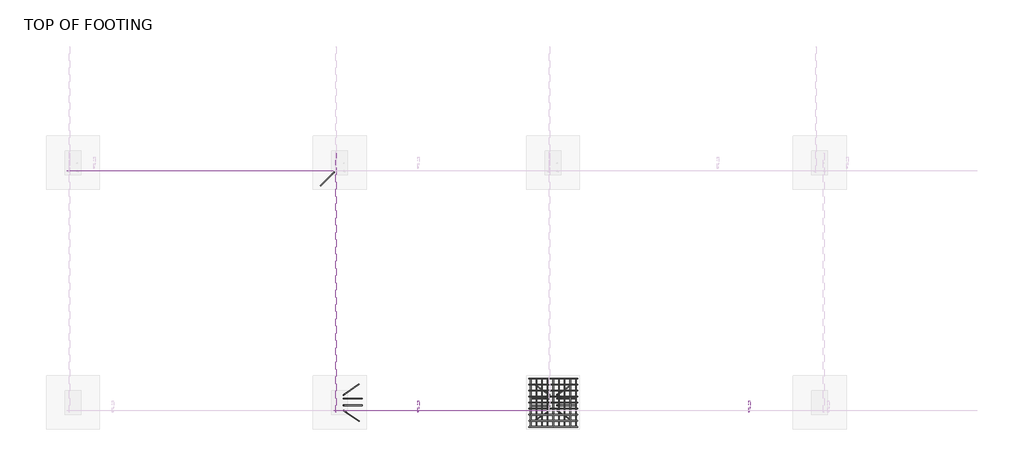
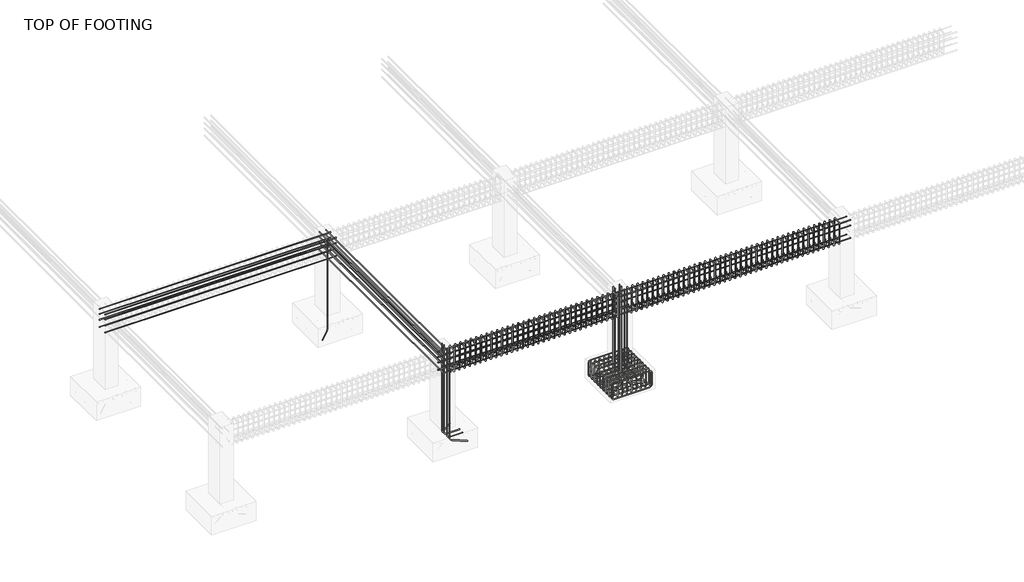
# One storey, part 3 of 13: 31 reinforcing bars.
"""IFC4 building model written with IfcOpenShell, lengths in millimetres."""

from ifc_helpers import new_model, si_unit, point, frame, origin, place, context, project, spatial, polyline, circle_curve, trimmed, segment, composite_curve, source, transform, mapped, element, save
from ifc_brep_helpers import swept_disk

model = new_model("IFC4")

# Units and contexts
model_context = context("Model", 3, world=origin())
ifc_project = project(units=[si_unit("LENGTHUNIT", "METRE", prefix="MILLI")], contexts=[model_context])

# Site, building, storey
site = spatial("IfcSite", under=ifc_project)
building = spatial("IfcBuilding", under=site)
storey = spatial("IfcBuildingStorey", under=building, Name="TOP OF FOOTING", Elevation=-1828.8)

# Reinforcing bars
placement = place(None, origin())
reinforcing_bar_shape = source(origin(), model_context, "Body", "SolidModel", [
    swept_disk(composite_curve([segment(polyline([(-3666.6498378, 3986.1851908, -2049.322685), (-3666.6498378, 3986.1851908, -2196.622685)]), True, "CONTINUOUS"), segment(trimmed(circle_curve(frame((-3712.9998378, 3986.1851908, -2196.622685), z_axis=(0.0, 1.0, 0.0), x_axis=(46.34999999999991, 0.0, 0.0)), 46.35), [point((-3666.6498378, 3986.1851908, -2196.622685))], [point((-3712.9998378, 3986.1851908, -2242.972685))], True, "CARTESIAN"), True, "CONTINUOUS"), segment(polyline([(-3712.9998378, 3986.1851908, -2242.972685), (-4527.5998378, 3986.1851908, -2242.972685)]), True, "CONTINUOUS"), segment(trimmed(circle_curve(frame((-4527.5998378, 3986.1851908, -2196.622685), z_axis=(0.0, 1.0, 0.0), x_axis=(0.0, 0.0, -46.350000000000364)), 46.35), [point((-4527.5998378, 3986.1851908, -2242.972685))], [point((-4573.9498378, 3986.1851908, -2196.622685))], True, "CARTESIAN"), True, "CONTINUOUS"), segment(polyline([(-4573.9498378, 3986.1851908, -2196.622685), (-4573.9498378, 3986.1851908, -2049.322685)]), True, "CONTINUOUS")], self_intersect=False), 6.35),
])
element("IfcReinforcingBar", 1, at=placement, inside=storey, context=model_context, shape_type="MappedRepresentation", body=[
    mapped(reinforcing_bar_shape, transform((0.0, 0.0, 0.0), x_axis=(1.0, 0.0, 0.0), y_axis=(0.0, 1.0, 0.0), z_axis=(0.0, 0.0, 1.0))),
    mapped(reinforcing_bar_shape, transform((0.0, -113.4125, 0.0), x_axis=(1.0, 0.0, 0.0), y_axis=(0.0, 1.0, 0.0), z_axis=(0.0, 0.0, 1.0))),
    mapped(reinforcing_bar_shape, transform((0.0, -226.825, 0.0), x_axis=(1.0, 0.0, 0.0), y_axis=(0.0, 1.0, 0.0), z_axis=(0.0, 0.0, 1.0))),
    mapped(reinforcing_bar_shape, transform((0.0, -340.2375, 0.0), x_axis=(1.0, 0.0, 0.0), y_axis=(0.0, 1.0, 0.0), z_axis=(0.0, 0.0, 1.0))),
    mapped(reinforcing_bar_shape, transform((0.0, -453.65, 0.0), x_axis=(1.0, 0.0, 0.0), y_axis=(0.0, 1.0, 0.0), z_axis=(0.0, 0.0, 1.0))),
    mapped(reinforcing_bar_shape, transform((0.0, -567.0625, 0.0), x_axis=(1.0, 0.0, 0.0), y_axis=(0.0, 1.0, 0.0), z_axis=(0.0, 0.0, 1.0))),
    mapped(reinforcing_bar_shape, transform((0.0, -680.475, 0.0), x_axis=(1.0, 0.0, 0.0), y_axis=(0.0, 1.0, 0.0), z_axis=(0.0, 0.0, 1.0))),
    mapped(reinforcing_bar_shape, transform((0.0, -793.8875, 0.0), x_axis=(1.0, 0.0, 0.0), y_axis=(0.0, 1.0, 0.0), z_axis=(0.0, 0.0, 1.0))),
    mapped(reinforcing_bar_shape, transform((0.0, -907.3, 0.0), x_axis=(1.0, 0.0, 0.0), y_axis=(0.0, 1.0, 0.0), z_axis=(0.0, 0.0, 1.0))),
])
reinforcing_bar_2_shape = source(origin(), model_context, "Body", "SolidModel", [
    swept_disk(composite_curve([segment(polyline([(-4573.9498378, 3986.1851908, -2051.3998363), (-4573.9498378, 3986.1851908, -1904.0998363)]), True, "CONTINUOUS"), segment(trimmed(circle_curve(frame((-4527.5998378, 3986.1851908, -1904.0998363), z_axis=(0.0, 1.0, 0.0), x_axis=(-46.349999999999454, 0.0, 0.0)), 46.35), [point((-4573.9498378, 3986.1851908, -1904.0998363))], [point((-4527.5998378, 3986.1851908, -1857.7498363))], True, "CARTESIAN"), True, "CONTINUOUS"), segment(polyline([(-4527.5998378, 3986.1851908, -1857.7498363), (-3712.9998378, 3986.1851908, -1857.7498363)]), True, "CONTINUOUS"), segment(trimmed(circle_curve(frame((-3712.9998378, 3986.1851908, -1904.0998363), z_axis=(0.0, 1.0, 0.0), x_axis=(0.0, 0.0, 46.350000000000136)), 46.35), [point((-3712.9998378, 3986.1851908, -1857.7498363))], [point((-3666.6498378, 3986.1851908, -1904.0998363))], True, "CARTESIAN"), True, "CONTINUOUS"), segment(polyline([(-3666.6498378, 3986.1851908, -1904.0998363), (-3666.6498378, 3986.1851908, -2051.3998363)]), True, "CONTINUOUS")], self_intersect=False), 6.35),
])
element("IfcReinforcingBar", 2, at=placement, inside=storey, context=model_context, shape_type="MappedRepresentation", body=[
    mapped(reinforcing_bar_2_shape, transform((0.0, 0.0, 0.0), x_axis=(1.0, 0.0, 0.0), y_axis=(0.0, 1.0, 0.0), z_axis=(0.0, 0.0, 1.0))),
    mapped(reinforcing_bar_2_shape, transform((0.0, -113.4125, 0.0), x_axis=(1.0, 0.0, 0.0), y_axis=(0.0, 1.0, 0.0), z_axis=(0.0, 0.0, 1.0))),
    mapped(reinforcing_bar_2_shape, transform((0.0, -226.825, 0.0), x_axis=(1.0, 0.0, 0.0), y_axis=(0.0, 1.0, 0.0), z_axis=(0.0, 0.0, 1.0))),
    mapped(reinforcing_bar_2_shape, transform((0.0, -340.2375, 0.0), x_axis=(1.0, 0.0, 0.0), y_axis=(0.0, 1.0, 0.0), z_axis=(0.0, 0.0, 1.0))),
    mapped(reinforcing_bar_2_shape, transform((0.0, -453.65, 0.0), x_axis=(1.0, 0.0, 0.0), y_axis=(0.0, 1.0, 0.0), z_axis=(0.0, 0.0, 1.0))),
    mapped(reinforcing_bar_2_shape, transform((0.0, -567.0625, 0.0), x_axis=(1.0, 0.0, 0.0), y_axis=(0.0, 1.0, 0.0), z_axis=(0.0, 0.0, 1.0))),
    mapped(reinforcing_bar_2_shape, transform((0.0, -680.475, 0.0), x_axis=(1.0, 0.0, 0.0), y_axis=(0.0, 1.0, 0.0), z_axis=(0.0, 0.0, 1.0))),
    mapped(reinforcing_bar_2_shape, transform((0.0, -793.8875, 0.0), x_axis=(1.0, 0.0, 0.0), y_axis=(0.0, 1.0, 0.0), z_axis=(0.0, 0.0, 1.0))),
    mapped(reinforcing_bar_2_shape, transform((0.0, -907.3, 0.0), x_axis=(1.0, 0.0, 0.0), y_axis=(0.0, 1.0, 0.0), z_axis=(0.0, 0.0, 1.0))),
])
reinforcing_bar_3_shape = source(origin(), model_context, "Body", "SolidModel", [
    swept_disk(composite_curve([segment(polyline([(-4542.4641345, 3986.1851908, -2025.081839), (-4542.4641345, 3986.1851908, -2172.381839)]), True, "CONTINUOUS"), segment(trimmed(circle_curve(frame((-4542.4641345, 3939.8351908, -2172.381839), z_axis=(-1.0, 0.0, 0.0), x_axis=(0.0, 46.34999999999991, 0.0)), 46.35), [point((-4542.4641345, 3986.1851908, -2172.381839))], [point((-4542.4641345, 3939.8351908, -2218.731839))], True, "CARTESIAN"), True, "CONTINUOUS"), segment(polyline([(-4542.4641345, 3939.8351908, -2218.731839), (-4542.4641345, 3125.2351908, -2218.731839)]), True, "CONTINUOUS"), segment(trimmed(circle_curve(frame((-4542.4641345, 3125.2351908, -2172.381839), z_axis=(-1.0, 0.0, 0.0), x_axis=(0.0, 0.0, -46.34999999999991)), 46.35), [point((-4542.4641345, 3125.2351908, -2218.731839))], [point((-4542.4641345, 3078.8851908, -2172.381839))], True, "CARTESIAN"), True, "CONTINUOUS"), segment(polyline([(-4542.4641345, 3078.8851908, -2172.381839), (-4542.4641345, 3078.8851908, -2025.081839)]), True, "CONTINUOUS")], self_intersect=False), 6.35),
])
element("IfcReinforcingBar", 3, at=placement, inside=storey, context=model_context, shape_type="MappedRepresentation", body=[
    mapped(reinforcing_bar_3_shape, transform((0.0, 0.0, 0.0), x_axis=(1.0, 0.0, 0.0), y_axis=(0.0, 1.0, 0.0), z_axis=(0.0, 0.0, 1.0))),
    mapped(reinforcing_bar_3_shape, transform((105.924033, 0.0, 0.0), x_axis=(1.0, 0.0, 0.0), y_axis=(0.0, 1.0, 0.0), z_axis=(0.0, 0.0, 1.0))),
    mapped(reinforcing_bar_3_shape, transform((211.8480661, 0.0, 0.0), x_axis=(1.0, 0.0, 0.0), y_axis=(0.0, 1.0, 0.0), z_axis=(0.0, 0.0, 1.0))),
    mapped(reinforcing_bar_3_shape, transform((317.7720991, 0.0, 0.0), x_axis=(1.0, 0.0, 0.0), y_axis=(0.0, 1.0, 0.0), z_axis=(0.0, 0.0, 1.0))),
    mapped(reinforcing_bar_3_shape, transform((423.6961321, 0.0, 0.0), x_axis=(1.0, 0.0, 0.0), y_axis=(0.0, 1.0, 0.0), z_axis=(0.0, 0.0, 1.0))),
    mapped(reinforcing_bar_3_shape, transform((529.6201652, 0.0, 0.0), x_axis=(1.0, 0.0, 0.0), y_axis=(0.0, 1.0, 0.0), z_axis=(0.0, 0.0, 1.0))),
    mapped(reinforcing_bar_3_shape, transform((635.5441982, 0.0, 0.0), x_axis=(1.0, 0.0, 0.0), y_axis=(0.0, 1.0, 0.0), z_axis=(0.0, 0.0, 1.0))),
    mapped(reinforcing_bar_3_shape, transform((741.4682312, 0.0, 0.0), x_axis=(1.0, 0.0, 0.0), y_axis=(0.0, 1.0, 0.0), z_axis=(0.0, 0.0, 1.0))),
    mapped(reinforcing_bar_3_shape, transform((847.3922643, 0.0, 0.0), x_axis=(1.0, 0.0, 0.0), y_axis=(0.0, 1.0, 0.0), z_axis=(0.0, 0.0, 1.0))),
])
reinforcing_bar_4_shape = source(origin(), model_context, "Body", "SolidModel", [
    swept_disk(composite_curve([segment(polyline([(-3695.0718702, 3986.1851908, -2069.0990329), (-3695.0718702, 3986.1851908, -1921.7990329)]), True, "CONTINUOUS"), segment(trimmed(circle_curve(frame((-3695.0718702, 3939.8351908, -1921.7990329), z_axis=(1.0, 0.0, 0.0), x_axis=(0.0, 46.34999999999991, 0.0)), 46.35), [point((-3695.0718702, 3986.1851908, -1921.7990329))], [point((-3695.0718702, 3939.8351908, -1875.4490329))], True, "CARTESIAN"), True, "CONTINUOUS"), segment(polyline([(-3695.0718702, 3939.8351908, -1875.4490329), (-3695.0718702, 3125.2351908, -1875.4490329)]), True, "CONTINUOUS"), segment(trimmed(circle_curve(frame((-3695.0718702, 3125.2351908, -1921.7990329), z_axis=(1.0, 0.0, 0.0), x_axis=(0.0, 0.0, 46.34999999999991)), 46.35), [point((-3695.0718702, 3125.2351908, -1875.4490329))], [point((-3695.0718702, 3078.8851908, -1921.7990329))], True, "CARTESIAN"), True, "CONTINUOUS"), segment(polyline([(-3695.0718702, 3078.8851908, -1921.7990329), (-3695.0718702, 3078.8851908, -2069.0990329)]), True, "CONTINUOUS")], self_intersect=False), 6.35),
])
element("IfcReinforcingBar", 4, at=placement, inside=storey, context=model_context, shape_type="MappedRepresentation", body=[
    mapped(reinforcing_bar_4_shape, transform((0.0, 0.0, 0.0), x_axis=(1.0, 0.0, 0.0), y_axis=(0.0, 1.0, 0.0), z_axis=(0.0, 0.0, 1.0))),
    mapped(reinforcing_bar_4_shape, transform((-105.924033, 0.0, 0.0), x_axis=(1.0, 0.0, 0.0), y_axis=(0.0, 1.0, 0.0), z_axis=(0.0, 0.0, 1.0))),
    mapped(reinforcing_bar_4_shape, transform((-211.8480661, 0.0, 0.0), x_axis=(1.0, 0.0, 0.0), y_axis=(0.0, 1.0, 0.0), z_axis=(0.0, 0.0, 1.0))),
    mapped(reinforcing_bar_4_shape, transform((-317.7720991, 0.0, 0.0), x_axis=(1.0, 0.0, 0.0), y_axis=(0.0, 1.0, 0.0), z_axis=(0.0, 0.0, 1.0))),
    mapped(reinforcing_bar_4_shape, transform((-423.6961321, 0.0, 0.0), x_axis=(1.0, 0.0, 0.0), y_axis=(0.0, 1.0, 0.0), z_axis=(0.0, 0.0, 1.0))),
    mapped(reinforcing_bar_4_shape, transform((-529.6201652, 0.0, 0.0), x_axis=(1.0, 0.0, 0.0), y_axis=(0.0, 1.0, 0.0), z_axis=(0.0, 0.0, 1.0))),
    mapped(reinforcing_bar_4_shape, transform((-635.5441982, 0.0, 0.0), x_axis=(1.0, 0.0, 0.0), y_axis=(0.0, 1.0, 0.0), z_axis=(0.0, 0.0, 1.0))),
    mapped(reinforcing_bar_4_shape, transform((-741.4682312, 0.0, 0.0), x_axis=(1.0, 0.0, 0.0), y_axis=(0.0, 1.0, 0.0), z_axis=(0.0, 0.0, 1.0))),
    mapped(reinforcing_bar_4_shape, transform((-847.3922643, 0.0, 0.0), x_axis=(1.0, 0.0, 0.0), y_axis=(0.0, 1.0, 0.0), z_axis=(0.0, 0.0, 1.0))),
])
element("IfcReinforcingBar", 5, at=placement, inside=storey, context=model_context, shape_type="SolidModel", body=[
    swept_disk(composite_curve([segment(polyline([(-8215.9186034, 7868.8851908, -40.0), (-8215.9186034, 7868.8851908, -2147.4714407)]), True, "CONTINUOUS"), segment(trimmed(circle_curve(frame((-8248.6930027, 7836.1107915, -2147.4714407), z_axis=(-0.7071067811865339, 0.7071067811865611, 0.0), x_axis=(32.77439930000037, 32.77439929999946, 0.0)), 46.35), [point((-8215.9186034, 7868.8851908, -2147.4714407))], [point((-8248.6930027, 7836.1107915, -2193.8214407))], True, "CARTESIAN"), True, "CONTINUOUS"), segment(polyline([(-8248.6930027, 7836.1107915, -2193.8214407), (-8482.6260737, 7602.1777205, -2193.8214407)]), True, "CONTINUOUS")], self_intersect=False), 6.35),
])
reinforcing_bar_5_shape = source(origin(), model_context, "Body", "SolidModel", [
    swept_disk(composite_curve([segment(polyline([(-4190.3202778, 3474.1031528, -40.0), (-4190.3202778, 3474.1031528, -2122.45)]), True, "CONTINUOUS"), segment(trimmed(circle_curve(frame((-4236.6702778, 3474.1031528, -2122.45), z_axis=(0.0, 1.0, 0.0), x_axis=(46.349999999999454, 0.0, 0.0)), 46.35), [point((-4190.3202778, 3474.1031528, -2122.45))], [point((-4236.6702778, 3474.1031528, -2168.8))], True, "CARTESIAN"), True, "CONTINUOUS"), segment(polyline([(-4236.6702778, 3474.1031528, -2168.8), (-4542.4641345, 3474.1031528, -2168.8)]), True, "CONTINUOUS")], self_intersect=False), 6.35),
])
element("IfcReinforcingBar", 6, at=placement, inside=storey, context=model_context, shape_type="MappedRepresentation", body=[
    mapped(reinforcing_bar_5_shape, transform((0.0, 0.0, 0.0), x_axis=(1.0, 0.0, 0.0), y_axis=(0.0, 1.0, 0.0), z_axis=(0.0, 0.0, 1.0))),
    mapped(reinforcing_bar_5_shape, transform((0.0, 133.432038, 0.0), x_axis=(1.0, 0.0, 0.0), y_axis=(0.0, 1.0, 0.0), z_axis=(0.0, 0.0, 1.0))),
])
element("IfcReinforcingBar", 7, at=placement, inside=storey, context=model_context, shape_type="SolidModel", body=[
    swept_disk(composite_curve([segment(polyline([(-4190.3202778, 3386.5851908, -40.0), (-4190.3202778, 3386.5851908, -2122.45)]), True, "CONTINUOUS"), segment(trimmed(circle_curve(frame((-4228.2879751, 3359.999923, -2122.45), z_axis=(-0.5735764363510439, 0.8191520442889934, 0.0), x_axis=(37.9676972999996, 26.58526780000011, 0.0)), 46.35), [point((-4190.3202778, 3386.5851908, -2122.45))], [point((-4228.2879751, 3359.999923, -2168.8))], True, "CARTESIAN"), True, "CONTINUOUS"), segment(polyline([(-4228.2879751, 3359.999923, -2168.8), (-4478.7796379, 3184.6037724, -2168.8)]), True, "CONTINUOUS")], self_intersect=False), 6.35),
])
element("IfcReinforcingBar", 8, at=placement, inside=storey, context=model_context, shape_type="SolidModel", body=[
    swept_disk(composite_curve([segment(polyline([(-4050.2793979, 3386.5851908, -40.0), (-4050.2793979, 3386.5851908, -2122.45)]), True, "CONTINUOUS"), segment(trimmed(circle_curve(frame((-4012.3117006, 3359.999923, -2122.45), z_axis=(-0.5735764363510439, -0.8191520442889934, 0.0), x_axis=(-37.9676972999996, 26.58526780000011, 0.0)), 46.35), [point((-4050.2793979, 3386.5851908, -2122.45))], [point((-4012.3117006, 3359.999923, -2168.8))], True, "CARTESIAN"), True, "CONTINUOUS"), segment(polyline([(-4012.3117006, 3359.999923, -2168.8), (-3761.8200378, 3184.6037724, -2168.8)]), True, "CONTINUOUS")], self_intersect=False), 6.35),
])
element("IfcReinforcingBar", 9, at=placement, inside=storey, context=model_context, shape_type="SolidModel", body=[
    swept_disk(composite_curve([segment(polyline([(-4190.3202778, 3678.4851908, -40.0), (-4190.3202778, 3678.4851908, -2122.45)]), True, "CONTINUOUS"), segment(trimmed(circle_curve(frame((-4228.2879751, 3705.0704586, -2122.45), z_axis=(0.5735764363510498, 0.8191520442889892, 0.0), x_axis=(37.9676972999996, -26.58526780000011, 0.0)), 46.35), [point((-4190.3202778, 3678.4851908, -2122.45))], [point((-4228.2879751, 3705.0704586, -2168.8))], True, "CARTESIAN"), True, "CONTINUOUS"), segment(polyline([(-4228.2879751, 3705.0704586, -2168.8), (-4478.7796379, 3880.4666092, -2168.8)]), True, "CONTINUOUS")], self_intersect=False), 6.35),
])
element("IfcReinforcingBar", 10, at=placement, inside=storey, context=model_context, shape_type="SolidModel", body=[
    swept_disk(composite_curve([segment(polyline([(-4050.2793979, 3678.4851908, -40.0), (-4050.2793979, 3678.4851908, -2122.45)]), True, "CONTINUOUS"), segment(trimmed(circle_curve(frame((-4012.3117006, 3705.0704586, -2122.45), z_axis=(0.573576436351038, -0.8191520442889975, 0.0), x_axis=(-37.9676972999996, -26.58526780000011, 0.0)), 46.35), [point((-4050.2793979, 3678.4851908, -2122.45))], [point((-4012.3117006, 3705.0704586, -2168.8))], True, "CARTESIAN"), True, "CONTINUOUS"), segment(polyline([(-4012.3117006, 3705.0704586, -2168.8), (-3761.8200378, 3880.4666092, -2168.8)]), True, "CONTINUOUS")], self_intersect=False), 6.35),
])
reinforcing_bar_6_shape = source(origin(), model_context, "Body", "SolidModel", [
    swept_disk(composite_curve([segment(polyline([(-4050.2793979, 3607.5351908, -40.0), (-4050.2793979, 3607.5351908, -2122.45)]), True, "CONTINUOUS"), segment(trimmed(circle_curve(frame((-4003.9293979, 3607.5351908, -2122.45), z_axis=(0.0, -1.0, 0.0), x_axis=(-46.34999999999991, 0.0, 0.0)), 46.35), [point((-4050.2793979, 3607.5351908, -2122.45))], [point((-4003.9293979, 3607.5351908, -2168.8))], True, "CARTESIAN"), True, "CONTINUOUS"), segment(polyline([(-4003.9293979, 3607.5351908, -2168.8), (-3697.3985869, 3607.5351908, -2168.8)]), True, "CONTINUOUS")], self_intersect=False), 6.35),
])
element("IfcReinforcingBar", 11, at=placement, inside=storey, context=model_context, shape_type="MappedRepresentation", body=[
    mapped(reinforcing_bar_6_shape, transform((0.0, 0.0, 0.0), x_axis=(1.0, 0.0, 0.0), y_axis=(0.0, 1.0, 0.0), z_axis=(0.0, 0.0, 1.0))),
    mapped(reinforcing_bar_6_shape, transform((0.0, -124.205444, 0.0), x_axis=(1.0, 0.0, 0.0), y_axis=(0.0, 1.0, 0.0), z_axis=(0.0, 0.0, 1.0))),
])
element("IfcReinforcingBar", 12, at=placement, inside=storey, context=model_context, shape_type="SolidModel", body=[
    swept_disk(composite_curve([segment(polyline([(-8050.2793979, 3386.5851908, -40.0), (-8050.2793979, 3386.5851908, -2122.45)]), True, "CONTINUOUS"), segment(trimmed(circle_curve(frame((-8012.3117006, 3359.999923, -2122.45), z_axis=(-0.5735764363510439, -0.8191520442889934, 0.0), x_axis=(-37.9676972999996, 26.58526780000011, 0.0)), 46.35), [point((-8050.2793979, 3386.5851908, -2122.45))], [point((-8012.3117006, 3359.999923, -2168.8))], True, "CARTESIAN"), True, "CONTINUOUS"), segment(polyline([(-8012.3117006, 3359.999923, -2168.8), (-7761.8200378, 3184.6037724, -2168.8)]), True, "CONTINUOUS")], self_intersect=False), 6.35),
])
element("IfcReinforcingBar", 13, at=placement, inside=storey, context=model_context, shape_type="SolidModel", body=[
    swept_disk(composite_curve([segment(polyline([(-8050.2793979, 3678.4851908, -40.0), (-8050.2793979, 3678.4851908, -2122.45)]), True, "CONTINUOUS"), segment(trimmed(circle_curve(frame((-8012.3117006, 3705.0704586, -2122.45), z_axis=(0.573576436351038, -0.8191520442889975, 0.0), x_axis=(-37.9676972999996, -26.58526780000011, 0.0)), 46.35), [point((-8050.2793979, 3678.4851908, -2122.45))], [point((-8012.3117006, 3705.0704586, -2168.8))], True, "CARTESIAN"), True, "CONTINUOUS"), segment(polyline([(-8012.3117006, 3705.0704586, -2168.8), (-7761.8200378, 3880.4666092, -2168.8)]), True, "CONTINUOUS")], self_intersect=False), 6.35),
])
reinforcing_bar_7_shape = source(origin(), model_context, "Body", "SolidModel", [
    swept_disk(composite_curve([segment(polyline([(-8050.2793979, 3607.5351908, -40.0), (-8050.2793979, 3607.5351908, -2122.45)]), True, "CONTINUOUS"), segment(trimmed(circle_curve(frame((-8003.9293979, 3607.5351908, -2122.45), z_axis=(0.0, -1.0, 0.0), x_axis=(-46.349999999999454, 0.0, 0.0)), 46.35), [point((-8050.2793979, 3607.5351908, -2122.45))], [point((-8003.9293979, 3607.5351908, -2168.8))], True, "CARTESIAN"), True, "CONTINUOUS"), segment(polyline([(-8003.9293979, 3607.5351908, -2168.8), (-7697.3985869, 3607.5351908, -2168.8)]), True, "CONTINUOUS")], self_intersect=False), 6.35),
])
element("IfcReinforcingBar", 14, at=placement, inside=storey, context=model_context, shape_type="MappedRepresentation", body=[
    mapped(reinforcing_bar_7_shape, transform((0.0, 0.0, 0.0), x_axis=(1.0, 0.0, 0.0), y_axis=(0.0, 1.0, 0.0), z_axis=(0.0, 0.0, 1.0))),
    mapped(reinforcing_bar_7_shape, transform((0.0, -124.205444, 0.0), x_axis=(1.0, 0.0, 0.0), y_axis=(0.0, 1.0, 0.0), z_axis=(0.0, 0.0, 1.0))),
])
reinforcing_bar_8_shape = source(origin(), model_context, "Body", "SolidModel", [
    swept_disk(composite_curve([segment(polyline([(-8047.9242736, 8217.5351908, -87.6047527), (-8047.9242736, 3347.5351908, -87.6047527)]), True, "CONTINUOUS")], self_intersect=False), 6.35),
])
element("IfcReinforcingBar", 15, at=placement, inside=storey, context=model_context, shape_type="MappedRepresentation", body=[
    mapped(reinforcing_bar_8_shape, transform((0.0, 0.0, 0.0), x_axis=(1.0, 0.0, 0.0), y_axis=(0.0, 1.0, 0.0), z_axis=(0.0, 0.0, 1.0))),
    mapped(reinforcing_bar_8_shape, transform((-144.710816, 0.0, 0.0), x_axis=(1.0, 0.0, 0.0), y_axis=(0.0, 1.0, 0.0), z_axis=(0.0, 0.0, 1.0))),
])
reinforcing_bar_9_shape = source(origin(), model_context, "Body", "SolidModel", [
    swept_disk(composite_curve([segment(polyline([(-8047.9242736, 8217.5351908, -212.6047527), (-8047.9242736, 3347.5351908, -212.6047527)]), True, "CONTINUOUS")], self_intersect=False), 6.35),
])
element("IfcReinforcingBar", 16, at=placement, inside=storey, context=model_context, shape_type="MappedRepresentation", body=[
    mapped(reinforcing_bar_9_shape, transform((0.0, 0.0, 0.0), x_axis=(1.0, 0.0, 0.0), y_axis=(0.0, 1.0, 0.0), z_axis=(0.0, 0.0, 1.0))),
    mapped(reinforcing_bar_9_shape, transform((-144.710816, 0.0, 0.0), x_axis=(1.0, 0.0, 0.0), y_axis=(0.0, 1.0, 0.0), z_axis=(0.0, 0.0, 1.0))),
])
reinforcing_bar_10_shape = source(origin(), model_context, "Body", "SolidModel", [
    swept_disk(composite_curve([segment(polyline([(-8047.9242736, 8217.5351908, -517.6047527), (-8047.9242736, 3347.5351908, -517.6047527)]), True, "CONTINUOUS")], self_intersect=False), 6.35),
])
element("IfcReinforcingBar", 17, at=placement, inside=storey, context=model_context, shape_type="MappedRepresentation", body=[
    mapped(reinforcing_bar_10_shape, transform((0.0, 0.0, 0.0), x_axis=(1.0, 0.0, 0.0), y_axis=(0.0, 1.0, 0.0), z_axis=(0.0, 0.0, 1.0))),
    mapped(reinforcing_bar_10_shape, transform((-144.710816, 0.0, 0.0), x_axis=(1.0, 0.0, 0.0), y_axis=(0.0, 1.0, 0.0), z_axis=(0.0, 0.0, 1.0))),
])
reinforcing_bar_11_shape = source(origin(), model_context, "Body", "SolidModel", [
    swept_disk(composite_curve([segment(polyline([(-8047.9242736, 8217.5351908, -347.6047527), (-8047.9242736, 3347.5351908, -347.6047527)]), True, "CONTINUOUS")], self_intersect=False), 6.35),
])
element("IfcReinforcingBar", 18, at=placement, inside=storey, context=model_context, shape_type="MappedRepresentation", body=[
    mapped(reinforcing_bar_11_shape, transform((0.0, 0.0, 0.0), x_axis=(1.0, 0.0, 0.0), y_axis=(0.0, 1.0, 0.0), z_axis=(0.0, 0.0, 1.0))),
    mapped(reinforcing_bar_11_shape, transform((-144.710816, 0.0, 0.0), x_axis=(1.0, 0.0, 0.0), y_axis=(0.0, 1.0, 0.0), z_axis=(0.0, 0.0, 1.0))),
])
reinforcing_bar_12_shape = source(origin(), model_context, "Body", "SolidModel", [
    swept_disk(composite_curve([segment(polyline([(-8010.2998378, 7885.1596265, -87.6047527), (-13230.2998378, 7885.1596265, -87.6047527)]), True, "CONTINUOUS")], self_intersect=False), 6.35),
])
element("IfcReinforcingBar", 19, at=placement, inside=storey, context=model_context, shape_type="MappedRepresentation", body=[
    mapped(reinforcing_bar_12_shape, transform((0.0, 0.0, 0.0), x_axis=(1.0, 0.0, 0.0), y_axis=(0.0, 1.0, 0.0), z_axis=(0.0, 0.0, 1.0))),
    mapped(reinforcing_bar_12_shape, transform((0.0, 219.710816, 0.0), x_axis=(1.0, 0.0, 0.0), y_axis=(0.0, 1.0, 0.0), z_axis=(0.0, 0.0, 1.0))),
])
reinforcing_bar_13_shape = source(origin(), model_context, "Body", "SolidModel", [
    swept_disk(composite_curve([segment(polyline([(-8010.2998378, 7885.1596265, -212.6047527), (-13230.2998378, 7885.1596265, -212.6047527)]), True, "CONTINUOUS")], self_intersect=False), 6.35),
])
element("IfcReinforcingBar", 20, at=placement, inside=storey, context=model_context, shape_type="MappedRepresentation", body=[
    mapped(reinforcing_bar_13_shape, transform((0.0, 0.0, 0.0), x_axis=(1.0, 0.0, 0.0), y_axis=(0.0, 1.0, 0.0), z_axis=(0.0, 0.0, 1.0))),
    mapped(reinforcing_bar_13_shape, transform((0.0, 219.710816, 0.0), x_axis=(1.0, 0.0, 0.0), y_axis=(0.0, 1.0, 0.0), z_axis=(0.0, 0.0, 1.0))),
])
reinforcing_bar_14_shape = source(origin(), model_context, "Body", "SolidModel", [
    swept_disk(composite_curve([segment(polyline([(-8010.2998378, 7885.1596265, -517.6047527), (-13230.2998378, 7885.1596265, -517.6047527)]), True, "CONTINUOUS")], self_intersect=False), 6.35),
])
element("IfcReinforcingBar", 21, at=placement, inside=storey, context=model_context, shape_type="MappedRepresentation", body=[
    mapped(reinforcing_bar_14_shape, transform((0.0, 0.0, 0.0), x_axis=(1.0, 0.0, 0.0), y_axis=(0.0, 1.0, 0.0), z_axis=(0.0, 0.0, 1.0))),
    mapped(reinforcing_bar_14_shape, transform((0.0, 219.710816, 0.0), x_axis=(1.0, 0.0, 0.0), y_axis=(0.0, 1.0, 0.0), z_axis=(0.0, 0.0, 1.0))),
])
reinforcing_bar_15_shape = source(origin(), model_context, "Body", "SolidModel", [
    swept_disk(composite_curve([segment(polyline([(-8010.2998378, 7885.1596265, -347.6047527), (-13230.2998378, 7885.1596265, -347.6047527)]), True, "CONTINUOUS")], self_intersect=False), 6.35),
])
element("IfcReinforcingBar", 22, at=placement, inside=storey, context=model_context, shape_type="MappedRepresentation", body=[
    mapped(reinforcing_bar_15_shape, transform((0.0, 0.0, 0.0), x_axis=(1.0, 0.0, 0.0), y_axis=(0.0, 1.0, 0.0), z_axis=(0.0, 0.0, 1.0))),
    mapped(reinforcing_bar_15_shape, transform((0.0, 219.710816, 0.0), x_axis=(1.0, 0.0, 0.0), y_axis=(0.0, 1.0, 0.0), z_axis=(0.0, 0.0, 1.0))),
])
reinforcing_bar_16_shape = source(origin(), model_context, "Body", "SolidModel", [
    swept_disk(composite_curve([segment(polyline([(723.3501622, 3496.2594254, -444.3886395), (723.3501622, 3552.0029884, -500.1322024)]), True, "CONTINUOUS"), segment(trimmed(circle_curve(frame((723.3501622, 3529.8351908, -522.3), z_axis=(-1.0, 0.0, 0.0), x_axis=(0.0, 22.167797600000085, 22.16779759999997)), 31.35), [point((723.3501622, 3552.0029884, -500.1322024))], [point((723.3501622, 3529.8351908, -553.65))], True, "CARTESIAN"), True, "CONTINUOUS"), segment(polyline([(723.3501622, 3529.8351908, -553.65), (723.3501622, 3385.2351908, -553.65)]), True, "CONTINUOUS"), segment(trimmed(circle_curve(frame((723.3501622, 3385.2351908, -522.3), z_axis=(-1.0, 0.0, 0.0), x_axis=(0.0, 0.0, -31.350000000000023)), 31.35), [point((723.3501622, 3385.2351908, -553.65))], [point((723.3501622, 3353.8851908, -522.3))], True, "CARTESIAN"), True, "CONTINUOUS"), segment(polyline([(723.3501622, 3353.8851908, -522.3), (723.3501622, 3353.8851908, -77.7)]), True, "CONTINUOUS"), segment(trimmed(circle_curve(frame((725.2671903, 3385.1765235, -77.7), z_axis=(-0.9981286353368323, 0.061149221750018364, 0.0), x_axis=(-1.9170281000000386, -31.291332699999657, 0.0)), 31.35), [point((723.3501622, 3353.8851908, -77.7))], [point((725.2671903, 3385.1765235, -46.35))], True, "CARTESIAN"), True, "CONTINUOUS"), segment(polyline([(725.2671903, 3385.1765235, -46.35), (734.1331341, 3529.8938581, -46.35)]), True, "CONTINUOUS"), segment(trimmed(circle_curve(frame((734.1331341, 3529.8938581, -77.7), z_axis=(-0.9981286353368323, 0.061149221750018364, 0.0), x_axis=(0.0, 0.0, 31.35)), 31.35), [point((734.1331341, 3529.8938581, -46.35))], [point((736.0501622, 3561.1851908, -77.7))], True, "CARTESIAN"), True, "CONTINUOUS"), segment(polyline([(736.0501622, 3561.1851908, -77.7), (736.0501622, 3561.1851908, -522.3)]), True, "CONTINUOUS"), segment(trimmed(circle_curve(frame((736.0501622, 3529.8351908, -522.3), z_axis=(-1.0, 0.0, 0.0), x_axis=(0.0, 31.34999999999991, 0.0)), 31.35), [point((736.0501622, 3561.1851908, -522.3))], [point((736.0501622, 3507.6673932, -544.4677976))], True, "CARTESIAN"), True, "CONTINUOUS"), segment(polyline([(736.0501622, 3507.6673932, -544.4677976), (736.0501622, 3451.9238303, -488.7242346)]), True, "CONTINUOUS")], self_intersect=False), 6.35),
])
element("IfcReinforcingBar", 23, at=placement, inside=storey, context=model_context, shape_type="MappedRepresentation", body=[
    mapped(reinforcing_bar_16_shape, transform((0.0, 0.0, 0.0), x_axis=(1.0, 0.0, 0.0), y_axis=(0.0, 1.0, 0.0), z_axis=(0.0, 0.0, 1.0))),
    mapped(reinforcing_bar_16_shape, transform((-117.1825, 0.0, 0.0), x_axis=(1.0, 0.0, 0.0), y_axis=(0.0, 1.0, 0.0), z_axis=(0.0, 0.0, 1.0))),
    mapped(reinforcing_bar_16_shape, transform((-234.365, 0.0, 0.0), x_axis=(1.0, 0.0, 0.0), y_axis=(0.0, 1.0, 0.0), z_axis=(0.0, 0.0, 1.0))),
    mapped(reinforcing_bar_16_shape, transform((-351.5475, 0.0, 0.0), x_axis=(1.0, 0.0, 0.0), y_axis=(0.0, 1.0, 0.0), z_axis=(0.0, 0.0, 1.0))),
    mapped(reinforcing_bar_16_shape, transform((-468.73, 0.0, 0.0), x_axis=(1.0, 0.0, 0.0), y_axis=(0.0, 1.0, 0.0), z_axis=(0.0, 0.0, 1.0))),
    mapped(reinforcing_bar_16_shape, transform((-585.9125, 0.0, 0.0), x_axis=(1.0, 0.0, 0.0), y_axis=(0.0, 1.0, 0.0), z_axis=(0.0, 0.0, 1.0))),
    mapped(reinforcing_bar_16_shape, transform((-703.095, 0.0, 0.0), x_axis=(1.0, 0.0, 0.0), y_axis=(0.0, 1.0, 0.0), z_axis=(0.0, 0.0, 1.0))),
    mapped(reinforcing_bar_16_shape, transform((-820.2775, 0.0, 0.0), x_axis=(1.0, 0.0, 0.0), y_axis=(0.0, 1.0, 0.0), z_axis=(0.0, 0.0, 1.0))),
    mapped(reinforcing_bar_16_shape, transform((-937.46, 0.0, 0.0), x_axis=(1.0, 0.0, 0.0), y_axis=(0.0, 1.0, 0.0), z_axis=(0.0, 0.0, 1.0))),
    mapped(reinforcing_bar_16_shape, transform((-1054.6425, 0.0, 0.0), x_axis=(1.0, 0.0, 0.0), y_axis=(0.0, 1.0, 0.0), z_axis=(0.0, 0.0, 1.0))),
    mapped(reinforcing_bar_16_shape, transform((-1171.825, 0.0, 0.0), x_axis=(1.0, 0.0, 0.0), y_axis=(0.0, 1.0, 0.0), z_axis=(0.0, 0.0, 1.0))),
    mapped(reinforcing_bar_16_shape, transform((-1289.0075, 0.0, 0.0), x_axis=(1.0, 0.0, 0.0), y_axis=(0.0, 1.0, 0.0), z_axis=(0.0, 0.0, 1.0))),
    mapped(reinforcing_bar_16_shape, transform((-1406.19, 0.0, 0.0), x_axis=(1.0, 0.0, 0.0), y_axis=(0.0, 1.0, 0.0), z_axis=(0.0, 0.0, 1.0))),
    mapped(reinforcing_bar_16_shape, transform((-1523.3725, 0.0, 0.0), x_axis=(1.0, 0.0, 0.0), y_axis=(0.0, 1.0, 0.0), z_axis=(0.0, 0.0, 1.0))),
    mapped(reinforcing_bar_16_shape, transform((-1640.555, 0.0, 0.0), x_axis=(1.0, 0.0, 0.0), y_axis=(0.0, 1.0, 0.0), z_axis=(0.0, 0.0, 1.0))),
    mapped(reinforcing_bar_16_shape, transform((-1757.7375, 0.0, 0.0), x_axis=(1.0, 0.0, 0.0), y_axis=(0.0, 1.0, 0.0), z_axis=(0.0, 0.0, 1.0))),
    mapped(reinforcing_bar_16_shape, transform((-1874.92, 0.0, 0.0), x_axis=(1.0, 0.0, 0.0), y_axis=(0.0, 1.0, 0.0), z_axis=(0.0, 0.0, 1.0))),
    mapped(reinforcing_bar_16_shape, transform((-1992.1025, 0.0, 0.0), x_axis=(1.0, 0.0, 0.0), y_axis=(0.0, 1.0, 0.0), z_axis=(0.0, 0.0, 1.0))),
    mapped(reinforcing_bar_16_shape, transform((-2109.285, 0.0, 0.0), x_axis=(1.0, 0.0, 0.0), y_axis=(0.0, 1.0, 0.0), z_axis=(0.0, 0.0, 1.0))),
    mapped(reinforcing_bar_16_shape, transform((-2226.4675, 0.0, 0.0), x_axis=(1.0, 0.0, 0.0), y_axis=(0.0, 1.0, 0.0), z_axis=(0.0, 0.0, 1.0))),
    mapped(reinforcing_bar_16_shape, transform((-2343.65, 0.0, 0.0), x_axis=(1.0, 0.0, 0.0), y_axis=(0.0, 1.0, 0.0), z_axis=(0.0, 0.0, 1.0))),
    mapped(reinforcing_bar_16_shape, transform((-2460.8325, 0.0, 0.0), x_axis=(1.0, 0.0, 0.0), y_axis=(0.0, 1.0, 0.0), z_axis=(0.0, 0.0, 1.0))),
    mapped(reinforcing_bar_16_shape, transform((-2578.015, 0.0, 0.0), x_axis=(1.0, 0.0, 0.0), y_axis=(0.0, 1.0, 0.0), z_axis=(0.0, 0.0, 1.0))),
    mapped(reinforcing_bar_16_shape, transform((-2695.1975, 0.0, 0.0), x_axis=(1.0, 0.0, 0.0), y_axis=(0.0, 1.0, 0.0), z_axis=(0.0, 0.0, 1.0))),
    mapped(reinforcing_bar_16_shape, transform((-2812.38, 0.0, 0.0), x_axis=(1.0, 0.0, 0.0), y_axis=(0.0, 1.0, 0.0), z_axis=(0.0, 0.0, 1.0))),
    mapped(reinforcing_bar_16_shape, transform((-2929.5625, 0.0, 0.0), x_axis=(1.0, 0.0, 0.0), y_axis=(0.0, 1.0, 0.0), z_axis=(0.0, 0.0, 1.0))),
    mapped(reinforcing_bar_16_shape, transform((-3046.745, 0.0, 0.0), x_axis=(1.0, 0.0, 0.0), y_axis=(0.0, 1.0, 0.0), z_axis=(0.0, 0.0, 1.0))),
    mapped(reinforcing_bar_16_shape, transform((-3163.9275, 0.0, 0.0), x_axis=(1.0, 0.0, 0.0), y_axis=(0.0, 1.0, 0.0), z_axis=(0.0, 0.0, 1.0))),
    mapped(reinforcing_bar_16_shape, transform((-3281.11, 0.0, 0.0), x_axis=(1.0, 0.0, 0.0), y_axis=(0.0, 1.0, 0.0), z_axis=(0.0, 0.0, 1.0))),
    mapped(reinforcing_bar_16_shape, transform((-3398.2925, 0.0, 0.0), x_axis=(1.0, 0.0, 0.0), y_axis=(0.0, 1.0, 0.0), z_axis=(0.0, 0.0, 1.0))),
    mapped(reinforcing_bar_16_shape, transform((-3515.475, 0.0, 0.0), x_axis=(1.0, 0.0, 0.0), y_axis=(0.0, 1.0, 0.0), z_axis=(0.0, 0.0, 1.0))),
    mapped(reinforcing_bar_16_shape, transform((-3632.6575, 0.0, 0.0), x_axis=(1.0, 0.0, 0.0), y_axis=(0.0, 1.0, 0.0), z_axis=(0.0, 0.0, 1.0))),
    mapped(reinforcing_bar_16_shape, transform((-3749.84, 0.0, 0.0), x_axis=(1.0, 0.0, 0.0), y_axis=(0.0, 1.0, 0.0), z_axis=(0.0, 0.0, 1.0))),
    mapped(reinforcing_bar_16_shape, transform((-3867.0225, 0.0, 0.0), x_axis=(1.0, 0.0, 0.0), y_axis=(0.0, 1.0, 0.0), z_axis=(0.0, 0.0, 1.0))),
    mapped(reinforcing_bar_16_shape, transform((-3984.205, 0.0, 0.0), x_axis=(1.0, 0.0, 0.0), y_axis=(0.0, 1.0, 0.0), z_axis=(0.0, 0.0, 1.0))),
    mapped(reinforcing_bar_16_shape, transform((-4101.3875, 0.0, 0.0), x_axis=(1.0, 0.0, 0.0), y_axis=(0.0, 1.0, 0.0), z_axis=(0.0, 0.0, 1.0))),
    mapped(reinforcing_bar_16_shape, transform((-4218.57, 0.0, 0.0), x_axis=(1.0, 0.0, 0.0), y_axis=(0.0, 1.0, 0.0), z_axis=(0.0, 0.0, 1.0))),
    mapped(reinforcing_bar_16_shape, transform((-4335.7525, 0.0, 0.0), x_axis=(1.0, 0.0, 0.0), y_axis=(0.0, 1.0, 0.0), z_axis=(0.0, 0.0, 1.0))),
    mapped(reinforcing_bar_16_shape, transform((-4452.935, 0.0, 0.0), x_axis=(1.0, 0.0, 0.0), y_axis=(0.0, 1.0, 0.0), z_axis=(0.0, 0.0, 1.0))),
    mapped(reinforcing_bar_16_shape, transform((-4570.1175, 0.0, 0.0), x_axis=(1.0, 0.0, 0.0), y_axis=(0.0, 1.0, 0.0), z_axis=(0.0, 0.0, 1.0))),
    mapped(reinforcing_bar_16_shape, transform((-4687.3, 0.0, 0.0), x_axis=(1.0, 0.0, 0.0), y_axis=(0.0, 1.0, 0.0), z_axis=(0.0, 0.0, 1.0))),
])
reinforcing_bar_17_shape = source(origin(), model_context, "Body", "SolidModel", [
    swept_disk(composite_curve([segment(polyline([(989.7001622, 3385.1596265, -87.6047527), (-4230.2998378, 3385.1596265, -87.6047527)]), True, "CONTINUOUS")], self_intersect=False), 6.35),
])
element("IfcReinforcingBar", 24, at=placement, inside=storey, context=model_context, shape_type="MappedRepresentation", body=[
    mapped(reinforcing_bar_17_shape, transform((0.0, 0.0, 0.0), x_axis=(1.0, 0.0, 0.0), y_axis=(0.0, 1.0, 0.0), z_axis=(0.0, 0.0, 1.0))),
    mapped(reinforcing_bar_17_shape, transform((0.0, 144.710816, 0.0), x_axis=(1.0, 0.0, 0.0), y_axis=(0.0, 1.0, 0.0), z_axis=(0.0, 0.0, 1.0))),
])
reinforcing_bar_18_shape = source(origin(), model_context, "Body", "SolidModel", [
    swept_disk(composite_curve([segment(polyline([(989.7001622, 3385.1596265, -212.6047527), (-4230.2998378, 3385.1596265, -212.6047527)]), True, "CONTINUOUS")], self_intersect=False), 6.35),
])
element("IfcReinforcingBar", 25, at=placement, inside=storey, context=model_context, shape_type="MappedRepresentation", body=[
    mapped(reinforcing_bar_18_shape, transform((0.0, 0.0, 0.0), x_axis=(1.0, 0.0, 0.0), y_axis=(0.0, 1.0, 0.0), z_axis=(0.0, 0.0, 1.0))),
    mapped(reinforcing_bar_18_shape, transform((0.0, 144.710816, 0.0), x_axis=(1.0, 0.0, 0.0), y_axis=(0.0, 1.0, 0.0), z_axis=(0.0, 0.0, 1.0))),
])
reinforcing_bar_19_shape = source(origin(), model_context, "Body", "SolidModel", [
    swept_disk(composite_curve([segment(polyline([(989.7001622, 3385.1596265, -517.6047527), (-4230.2998378, 3385.1596265, -517.6047527)]), True, "CONTINUOUS")], self_intersect=False), 6.35),
])
element("IfcReinforcingBar", 26, at=placement, inside=storey, context=model_context, shape_type="MappedRepresentation", body=[
    mapped(reinforcing_bar_19_shape, transform((0.0, 0.0, 0.0), x_axis=(1.0, 0.0, 0.0), y_axis=(0.0, 1.0, 0.0), z_axis=(0.0, 0.0, 1.0))),
    mapped(reinforcing_bar_19_shape, transform((0.0, 144.710816, 0.0), x_axis=(1.0, 0.0, 0.0), y_axis=(0.0, 1.0, 0.0), z_axis=(0.0, 0.0, 1.0))),
])
reinforcing_bar_20_shape = source(origin(), model_context, "Body", "SolidModel", [
    swept_disk(composite_curve([segment(polyline([(-4276.6498378, 3496.2594254, -444.3886395), (-4276.6498378, 3552.0029884, -500.1322024)]), True, "CONTINUOUS"), segment(trimmed(circle_curve(frame((-4276.6498378, 3529.8351908, -522.3), z_axis=(-1.0, 0.0, 0.0), x_axis=(0.0, 22.167797600000085, 22.16779759999997)), 31.35), [point((-4276.6498378, 3552.0029884, -500.1322024))], [point((-4276.6498378, 3529.8351908, -553.65))], True, "CARTESIAN"), True, "CONTINUOUS"), segment(polyline([(-4276.6498378, 3529.8351908, -553.65), (-4276.6498378, 3385.2351908, -553.65)]), True, "CONTINUOUS"), segment(trimmed(circle_curve(frame((-4276.6498378, 3385.2351908, -522.3), z_axis=(-1.0, 0.0, 0.0), x_axis=(0.0, 0.0, -31.350000000000023)), 31.35), [point((-4276.6498378, 3385.2351908, -553.65))], [point((-4276.6498378, 3353.8851908, -522.3))], True, "CARTESIAN"), True, "CONTINUOUS"), segment(polyline([(-4276.6498378, 3353.8851908, -522.3), (-4276.6498378, 3353.8851908, -77.7)]), True, "CONTINUOUS"), segment(trimmed(circle_curve(frame((-4274.7328097, 3385.1765235, -77.7), z_axis=(-0.9981286353368323, 0.06114922175001836, 0.0), x_axis=(-1.9170280999996976, -31.291332699999657, 0.0)), 31.35), [point((-4276.6498378, 3353.8851908, -77.7))], [point((-4274.7328097, 3385.1765235, -46.35))], True, "CARTESIAN"), True, "CONTINUOUS"), segment(polyline([(-4274.7328097, 3385.1765235, -46.35), (-4265.8668659, 3529.8938581, -46.35)]), True, "CONTINUOUS"), segment(trimmed(circle_curve(frame((-4265.8668659, 3529.8938581, -77.7), z_axis=(-0.9981286353368323, 0.06114922175001836, 0.0), x_axis=(0.0, 0.0, 31.35)), 31.35), [point((-4265.8668659, 3529.8938581, -46.35))], [point((-4263.9498378, 3561.1851908, -77.7))], True, "CARTESIAN"), True, "CONTINUOUS"), segment(polyline([(-4263.9498378, 3561.1851908, -77.7), (-4263.9498378, 3561.1851908, -522.3)]), True, "CONTINUOUS"), segment(trimmed(circle_curve(frame((-4263.9498378, 3529.8351908, -522.3), z_axis=(-1.0, 0.0, 0.0), x_axis=(0.0, 31.34999999999991, 0.0)), 31.35), [point((-4263.9498378, 3561.1851908, -522.3))], [point((-4263.9498378, 3507.6673932, -544.4677976))], True, "CARTESIAN"), True, "CONTINUOUS"), segment(polyline([(-4263.9498378, 3507.6673932, -544.4677976), (-4263.9498378, 3451.9238303, -488.7242346)]), True, "CONTINUOUS")], self_intersect=False), 6.35),
])
element("IfcReinforcingBar", 27, at=placement, inside=storey, context=model_context, shape_type="MappedRepresentation", body=[
    mapped(reinforcing_bar_20_shape, transform((0.0, 0.0, 0.0), x_axis=(1.0, 0.0, 0.0), y_axis=(0.0, 1.0, 0.0), z_axis=(0.0, 0.0, 1.0))),
    mapped(reinforcing_bar_20_shape, transform((-118.9451613, 0.0, 0.0), x_axis=(1.0, 0.0, 0.0), y_axis=(0.0, 1.0, 0.0), z_axis=(0.0, 0.0, 1.0))),
    mapped(reinforcing_bar_20_shape, transform((-237.8903226, 0.0, 0.0), x_axis=(1.0, 0.0, 0.0), y_axis=(0.0, 1.0, 0.0), z_axis=(0.0, 0.0, 1.0))),
    mapped(reinforcing_bar_20_shape, transform((-356.8354839, 0.0, 0.0), x_axis=(1.0, 0.0, 0.0), y_axis=(0.0, 1.0, 0.0), z_axis=(0.0, 0.0, 1.0))),
    mapped(reinforcing_bar_20_shape, transform((-475.7806452, 0.0, 0.0), x_axis=(1.0, 0.0, 0.0), y_axis=(0.0, 1.0, 0.0), z_axis=(0.0, 0.0, 1.0))),
    mapped(reinforcing_bar_20_shape, transform((-594.7258065, 0.0, 0.0), x_axis=(1.0, 0.0, 0.0), y_axis=(0.0, 1.0, 0.0), z_axis=(0.0, 0.0, 1.0))),
    mapped(reinforcing_bar_20_shape, transform((-713.6709677, 0.0, 0.0), x_axis=(1.0, 0.0, 0.0), y_axis=(0.0, 1.0, 0.0), z_axis=(0.0, 0.0, 1.0))),
    mapped(reinforcing_bar_20_shape, transform((-832.616129, 0.0, 0.0), x_axis=(1.0, 0.0, 0.0), y_axis=(0.0, 1.0, 0.0), z_axis=(0.0, 0.0, 1.0))),
    mapped(reinforcing_bar_20_shape, transform((-951.5612903, 0.0, 0.0), x_axis=(1.0, 0.0, 0.0), y_axis=(0.0, 1.0, 0.0), z_axis=(0.0, 0.0, 1.0))),
    mapped(reinforcing_bar_20_shape, transform((-1070.5064516, 0.0, 0.0), x_axis=(1.0, 0.0, 0.0), y_axis=(0.0, 1.0, 0.0), z_axis=(0.0, 0.0, 1.0))),
    mapped(reinforcing_bar_20_shape, transform((-1189.4516129, 0.0, 0.0), x_axis=(1.0, 0.0, 0.0), y_axis=(0.0, 1.0, 0.0), z_axis=(0.0, 0.0, 1.0))),
    mapped(reinforcing_bar_20_shape, transform((-1308.3967742, 0.0, 0.0), x_axis=(1.0, 0.0, 0.0), y_axis=(0.0, 1.0, 0.0), z_axis=(0.0, 0.0, 1.0))),
    mapped(reinforcing_bar_20_shape, transform((-1427.3419355, 0.0, 0.0), x_axis=(1.0, 0.0, 0.0), y_axis=(0.0, 1.0, 0.0), z_axis=(0.0, 0.0, 1.0))),
    mapped(reinforcing_bar_20_shape, transform((-1546.2870968, 0.0, 0.0), x_axis=(1.0, 0.0, 0.0), y_axis=(0.0, 1.0, 0.0), z_axis=(0.0, 0.0, 1.0))),
    mapped(reinforcing_bar_20_shape, transform((-1665.2322581, 0.0, 0.0), x_axis=(1.0, 0.0, 0.0), y_axis=(0.0, 1.0, 0.0), z_axis=(0.0, 0.0, 1.0))),
    mapped(reinforcing_bar_20_shape, transform((-1784.1774194, 0.0, 0.0), x_axis=(1.0, 0.0, 0.0), y_axis=(0.0, 1.0, 0.0), z_axis=(0.0, 0.0, 1.0))),
    mapped(reinforcing_bar_20_shape, transform((-1903.1225806, 0.0, 0.0), x_axis=(1.0, 0.0, 0.0), y_axis=(0.0, 1.0, 0.0), z_axis=(0.0, 0.0, 1.0))),
    mapped(reinforcing_bar_20_shape, transform((-2022.0677419, 0.0, 0.0), x_axis=(1.0, 0.0, 0.0), y_axis=(0.0, 1.0, 0.0), z_axis=(0.0, 0.0, 1.0))),
    mapped(reinforcing_bar_20_shape, transform((-2141.0129032, 0.0, 0.0), x_axis=(1.0, 0.0, 0.0), y_axis=(0.0, 1.0, 0.0), z_axis=(0.0, 0.0, 1.0))),
    mapped(reinforcing_bar_20_shape, transform((-2259.9580645, 0.0, 0.0), x_axis=(1.0, 0.0, 0.0), y_axis=(0.0, 1.0, 0.0), z_axis=(0.0, 0.0, 1.0))),
    mapped(reinforcing_bar_20_shape, transform((-2378.9032258, 0.0, 0.0), x_axis=(1.0, 0.0, 0.0), y_axis=(0.0, 1.0, 0.0), z_axis=(0.0, 0.0, 1.0))),
    mapped(reinforcing_bar_20_shape, transform((-2497.8483871, 0.0, 0.0), x_axis=(1.0, 0.0, 0.0), y_axis=(0.0, 1.0, 0.0), z_axis=(0.0, 0.0, 1.0))),
    mapped(reinforcing_bar_20_shape, transform((-2616.7935484, 0.0, 0.0), x_axis=(1.0, 0.0, 0.0), y_axis=(0.0, 1.0, 0.0), z_axis=(0.0, 0.0, 1.0))),
    mapped(reinforcing_bar_20_shape, transform((-2735.7387097, 0.0, 0.0), x_axis=(1.0, 0.0, 0.0), y_axis=(0.0, 1.0, 0.0), z_axis=(0.0, 0.0, 1.0))),
    mapped(reinforcing_bar_20_shape, transform((-2854.683871, 0.0, 0.0), x_axis=(1.0, 0.0, 0.0), y_axis=(0.0, 1.0, 0.0), z_axis=(0.0, 0.0, 1.0))),
    mapped(reinforcing_bar_20_shape, transform((-2973.6290323, 0.0, 0.0), x_axis=(1.0, 0.0, 0.0), y_axis=(0.0, 1.0, 0.0), z_axis=(0.0, 0.0, 1.0))),
    mapped(reinforcing_bar_20_shape, transform((-3092.5741935, 0.0, 0.0), x_axis=(1.0, 0.0, 0.0), y_axis=(0.0, 1.0, 0.0), z_axis=(0.0, 0.0, 1.0))),
    mapped(reinforcing_bar_20_shape, transform((-3211.5193548, 0.0, 0.0), x_axis=(1.0, 0.0, 0.0), y_axis=(0.0, 1.0, 0.0), z_axis=(0.0, 0.0, 1.0))),
    mapped(reinforcing_bar_20_shape, transform((-3330.4645161, 0.0, 0.0), x_axis=(1.0, 0.0, 0.0), y_axis=(0.0, 1.0, 0.0), z_axis=(0.0, 0.0, 1.0))),
    mapped(reinforcing_bar_20_shape, transform((-3449.4096774, 0.0, 0.0), x_axis=(1.0, 0.0, 0.0), y_axis=(0.0, 1.0, 0.0), z_axis=(0.0, 0.0, 1.0))),
    mapped(reinforcing_bar_20_shape, transform((-3568.3548387, 0.0, 0.0), x_axis=(1.0, 0.0, 0.0), y_axis=(0.0, 1.0, 0.0), z_axis=(0.0, 0.0, 1.0))),
    mapped(reinforcing_bar_20_shape, transform((-3687.3, 0.0, 0.0), x_axis=(1.0, 0.0, 0.0), y_axis=(0.0, 1.0, 0.0), z_axis=(0.0, 0.0, 1.0))),
])
reinforcing_bar_21_shape = source(origin(), model_context, "Body", "SolidModel", [
    swept_disk(composite_curve([segment(polyline([(-4010.2998378, 3385.1596265, -87.6047527), (-8230.2998378, 3385.1596265, -87.6047527)]), True, "CONTINUOUS")], self_intersect=False), 6.35),
])
element("IfcReinforcingBar", 28, at=placement, inside=storey, context=model_context, shape_type="MappedRepresentation", body=[
    mapped(reinforcing_bar_21_shape, transform((0.0, 0.0, 0.0), x_axis=(1.0, 0.0, 0.0), y_axis=(0.0, 1.0, 0.0), z_axis=(0.0, 0.0, 1.0))),
    mapped(reinforcing_bar_21_shape, transform((0.0, 144.710816, 0.0), x_axis=(1.0, 0.0, 0.0), y_axis=(0.0, 1.0, 0.0), z_axis=(0.0, 0.0, 1.0))),
])
reinforcing_bar_22_shape = source(origin(), model_context, "Body", "SolidModel", [
    swept_disk(composite_curve([segment(polyline([(-4010.2998378, 3385.1596265, -212.6047527), (-8230.2998378, 3385.1596265, -212.6047527)]), True, "CONTINUOUS")], self_intersect=False), 6.35),
])
element("IfcReinforcingBar", 29, at=placement, inside=storey, context=model_context, shape_type="MappedRepresentation", body=[
    mapped(reinforcing_bar_22_shape, transform((0.0, 0.0, 0.0), x_axis=(1.0, 0.0, 0.0), y_axis=(0.0, 1.0, 0.0), z_axis=(0.0, 0.0, 1.0))),
    mapped(reinforcing_bar_22_shape, transform((0.0, 144.710816, 0.0), x_axis=(1.0, 0.0, 0.0), y_axis=(0.0, 1.0, 0.0), z_axis=(0.0, 0.0, 1.0))),
])
reinforcing_bar_23_shape = source(origin(), model_context, "Body", "SolidModel", [
    swept_disk(composite_curve([segment(polyline([(-4010.2998378, 3385.1596265, -517.6047527), (-8230.2998378, 3385.1596265, -517.6047527)]), True, "CONTINUOUS")], self_intersect=False), 6.35),
])
element("IfcReinforcingBar", 30, at=placement, inside=storey, context=model_context, shape_type="MappedRepresentation", body=[
    mapped(reinforcing_bar_23_shape, transform((0.0, 0.0, 0.0), x_axis=(1.0, 0.0, 0.0), y_axis=(0.0, 1.0, 0.0), z_axis=(0.0, 0.0, 1.0))),
    mapped(reinforcing_bar_23_shape, transform((0.0, 144.710816, 0.0), x_axis=(1.0, 0.0, 0.0), y_axis=(0.0, 1.0, 0.0), z_axis=(0.0, 0.0, 1.0))),
])
reinforcing_bar_24_shape = source(origin(), model_context, "Body", "SolidModel", [
    swept_disk(composite_curve([segment(polyline([(-4010.2998378, 3385.1596265, -347.6047527), (-8230.2998378, 3385.1596265, -347.6047527)]), True, "CONTINUOUS")], self_intersect=False), 6.35),
])
element("IfcReinforcingBar", 31, at=placement, inside=storey, context=model_context, shape_type="MappedRepresentation", body=[
    mapped(reinforcing_bar_24_shape, transform((0.0, 0.0, 0.0), x_axis=(1.0, 0.0, 0.0), y_axis=(0.0, 1.0, 0.0), z_axis=(0.0, 0.0, 1.0))),
    mapped(reinforcing_bar_24_shape, transform((0.0, 144.710816, 0.0), x_axis=(1.0, 0.0, 0.0), y_axis=(0.0, 1.0, 0.0), z_axis=(0.0, 0.0, 1.0))),
])

save(model, "model.ifc")

# Revit data of these elements
# Elements 1, 2, 3, 4, 5, 6, 7, 8, 9, 10, 11, 12, 13, 14, 15, 16, 17, 18, 19, 20, 21, 22, 23, 24, 25, 26, 27, 28, 29, 30, 31 (IfcReinforcingBar)
#   Phase Created = New Construction
